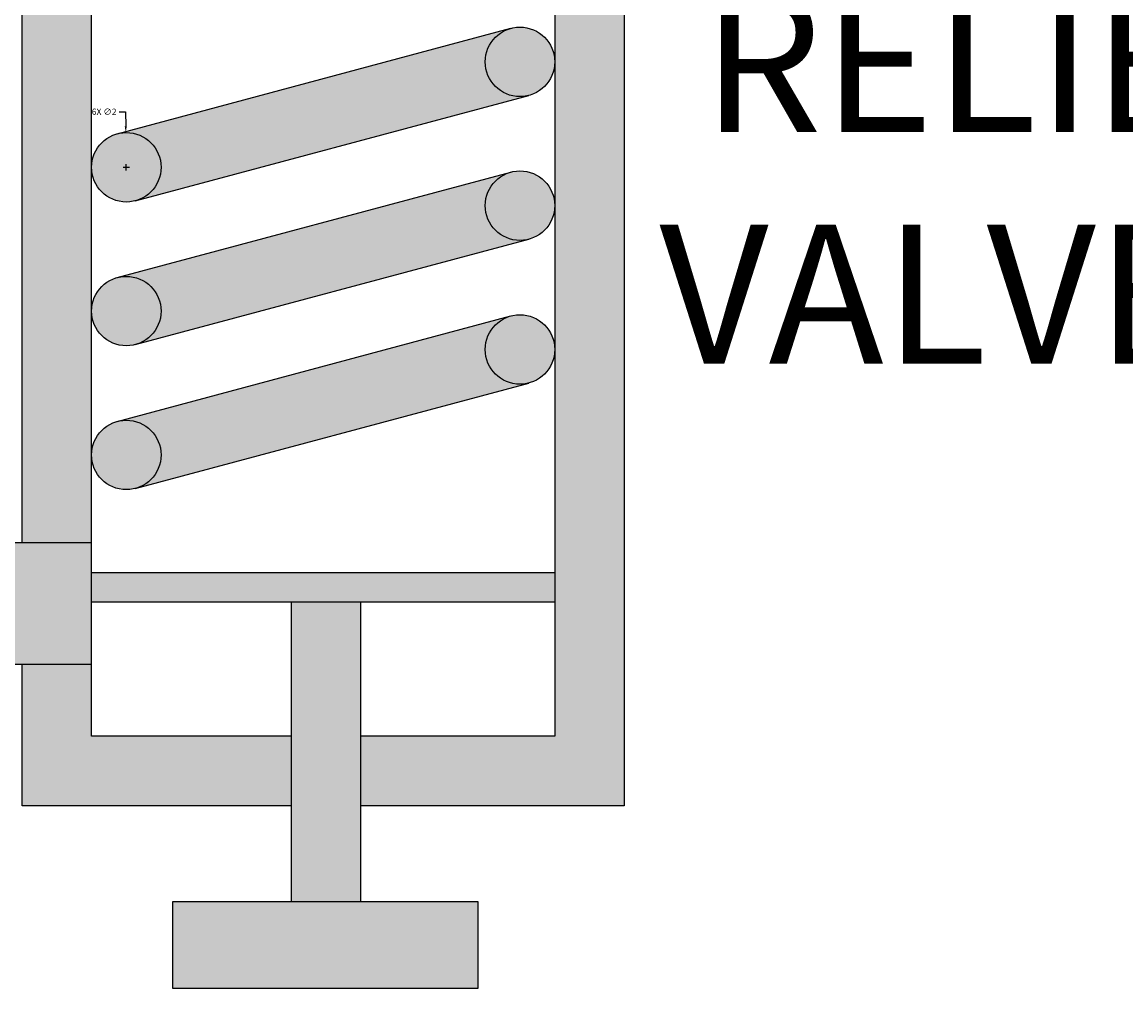
# Model space of a CAD drawing. Units: millimetres. Extents: x -11 to 280, y -4 to 208.
# Tile 23 of 55: x 119 to 150, y 61 to 89. Entities that reach past the tile are written whole.
import ezdxf

# ---------------------------------------------------------------- set-up
doc = ezdxf.new("R2010")
doc.units = ezdxf.units.MM
for name, color, linetype, lineweight in [('M-ANNO-TEXT', 7, 'Continuous', 18), ('M-DIMS', 2, 'Continuous', 18), ('M-HYDR-RETN', 7, 'Continuous', 25), ('M-HYDR-VALV', 7, 'Continuous', 25), ('M-HYDR-VALV-PATT', 252, 'Continuous', 13)]:
    doc.layers.add(name, color=color, linetype=linetype, lineweight=lineweight)
doc.layers.add('M-HYDR-RETN-PATT', color=114, linetype='Continuous', lineweight=13, true_color=0x139b48)
doc.styles.get("Standard").update_dxf_attribs({"font": 'arial.ttf'})
doc.dimstyles.get("Standard").update_dxf_attribs({"dimtxt": 0.18, "dimasz": 0.18, "dimexe": 0.18, "dimexo": 0.0625, "dimgap": 0.09, "dimtad": 0, "dimtih": 1, "dimtoh": 1, "dimdec": 4, "dimzin": 0, "dimdsep": 46, "dimtxsty": 'Standard', "dimcen": 0.09, "dimadec": 0, "dimazin": 0, "dimtfac": 1, "dimtdec": 4, "dimtofl": 0, "dimtmove": 0, "dimatfit": 3, "dimfxl": 1, "dimtolj": 1, "dimtzin": 0, "dimarcsym": 0})

# ---------------------------------------------------------------- blocks, each defined once
blk = doc.blocks.new('*D4')
at = {"layer": 'Defpoints', "color": 0, "transparency": 16777216}
for p in [(4.763, 84.426), (266.035, 51.733), (266.035, -3.415)]:
    blk.add_point(p, dxfattribs=at)
at = {"layer": 'M-DIMS', "color": 0, "lineweight": -2, "transparency": 16777216}
for p, q in [((4.763, 84.364), (4.763, -3.595)), ((266.035, 51.67), (266.035, -3.595)), ((4.943, -3.415), (134.934, -3.415)), ((265.855, -3.415), (135.864, -3.415))]:
    blk.add_line(p, q, dxfattribs=at)
at = {"layer": 'M-DIMS', "color": 0, "transparency": 16777216}
for points in [[(4.943, -3.385), (4.943, -3.445), (4.763, -3.415)], [(265.855, -3.385), (265.855, -3.445), (266.035, -3.415)]]:
    blk.add_solid(points, dxfattribs=at)
at = {"layer": 'M-DIMS', "color": 0, "transparency": 16777216, "insert": (135.399, -3.415), "char_height": 0.18, "attachment_point": 5}
blk.add_mtext('\\A1;261.27', dxfattribs=at)
blk = doc.blocks.new('*D5')
at = {"layer": 'Defpoints', "color": 0, "transparency": 16777216}
for p in [(24.759, 192.645), (-10.087, 11.435), (261.686, 11.435)]:
    blk.add_point(p, dxfattribs=at)
at = {"layer": 'M-DIMS', "color": 0, "lineweight": -2, "transparency": 16777216}
for p, q in [((24.696, 192.645), (-10.267, 192.645)), ((-10.087, 192.465), (-10.087, 102.222)), ((-10.087, 11.615), (-10.087, 101.858)), ((261.624, 11.435), (-10.267, 11.435))]:
    blk.add_line(p, q, dxfattribs=at)
at = {"layer": 'M-DIMS', "color": 0, "transparency": 16777216}
for points in [[(-10.117, 192.465), (-10.057, 192.465), (-10.087, 192.645)], [(-10.117, 11.615), (-10.057, 11.615), (-10.087, 11.435)]]:
    blk.add_solid(points, dxfattribs=at)
at = {"layer": 'M-DIMS', "color": 0, "transparency": 16777216, "insert": (-10.087, 102.04), "char_height": 0.18, "attachment_point": 5}
blk.add_mtext('\\A1;181.2', dxfattribs=at)
blk = doc.blocks.new('*D32')
at = {"layer": 'Defpoints', "color": 0, "transparency": 16777216}
for p in [(121.5, 86.206), (121.527, 84.206)]:
    blk.add_point(p, dxfattribs=at)
at = {"layer": 'M-DIMS', "color": 0, "lineweight": -2, "transparency": 16777216}
for p, q in [((121.312, 86.806), (121.492, 86.806)), ((121.492, 86.806), (121.497, 86.386)), ((121.424, 85.206), (121.604, 85.206)), ((121.514, 85.116), (121.514, 85.296))]:
    blk.add_line(p, q, dxfattribs=at)
at = {"layer": 'M-DIMS', "color": 0, "transparency": 16777216}
blk.add_solid([(121.527, 86.387), (121.467, 86.386), (121.5, 86.206)], dxfattribs=at)
at = {"layer": 'M-DIMS', "color": 0, "transparency": 16777216, "insert": (120.877, 86.806), "char_height": 0.18, "attachment_point": 5}
blk.add_mtext('\\A1;6X ∅2', dxfattribs=at)

msp = doc.modelspace()

# ---------------------------------------------------------------- hatches: boundary and pattern name
at = {"layer": 'M-HYDR-RETN-PATT'}
h = msp.add_hatch(color=256, dxfattribs=at)
h.set_gradient(color1=(19, 155, 72), color2=(19, 155, 72), tint=1)
h.paths.add_polyline_path([(17.9701, 159.0814), (29.2015, 159.0814), (29.2015, 162.5814), (14.4701, 162.5814), (14.4701, 98.0213), (17.9701, 98.0213)])
h.paths.add_polyline_path([(17.9701, 84.4261), (14.4701, 84.4261), (14.4701, 54.3099), (156.2446, 54.3099), (156.2446, 57.8099), (17.9701, 57.8099)])
h.paths.add_polyline_path([(120.5137, 74.3991), (17.9701, 74.3991), (17.9701, 70.8991), (120.5137, 70.8991)], flags=17)
h.paths.add_polyline_path([(184.7092, 75.04, 0.4142136), (179.7092, 80.04), (156.2446, 80.04), (156.2446, 57.8099), (156.2446, 54.3099), (156.2446, 43.5991), (159.7446, 43.5991), (159.7446, 57.8099), (159.7446, 76.54), (176.2092, 76.54, -0.4142136), (181.2092, 71.54), (181.2092, 57.8099), (159.7446, 57.8099), (159.7446, 54.3099), (184.7092, 54.3099)])
at = {"layer": 'M-HYDR-VALV-PATT'}
h = msp.add_hatch(color=256, dxfattribs=at)
h.set_gradient(color1=(153, 153, 0), color2=(153, 153, 0), tint=1)
h.paths.add_polyline_path([(135.8437, 96.4849), (128.8433, 96.4849), (128.8433, 94.4849), (133.8437, 94.4849), (133.8437, 68.8227), (128.2568, 68.8227), (128.2568, 66.8227), (135.8437, 66.8227)])
h.paths.add_polyline_path([(126.2568, 68.8227), (120.5137, 68.8227), (120.5137, 70.8991), (118.5137, 70.8991), (118.5137, 66.8227), (126.2568, 66.8227)])
h.paths.add_polyline_path([(120.5137, 94.4849), (125.3433, 94.4849), (125.3433, 96.4849), (118.5137, 96.4849), (118.5137, 74.3991), (120.5137, 74.3991)])
h.paths.add_polyline_path([(128.2568, 72.69), (126.2568, 72.69), (126.2568, 64.0664), (128.2568, 64.0664)])
h.paths.add_polyline_path([(131.6327, 64.0664), (122.8484, 64.0664), (122.8484, 61.5587), (131.6327, 61.5587)])
h.paths.add_polyline_path([(133.8437, 73.5419), (120.5137, 73.5419), (120.5137, 72.69), (133.8437, 72.69)])
h = msp.add_hatch(color=256, dxfattribs=at)
h.set_gradient(color1=(153, 27, 30), color2=(153, 27, 30), tint=1)
h.paths.add_polyline_path([(131.8437, 88.2421, -0.3394543), (132.5849, 89.208), (121.2548, 86.1721, -0.4931454), (122.5137, 85.2062, -0.3394543), (121.7725, 84.2403), (133.1025, 87.2762, -0.4931454)])
h.paths.add_polyline_path([(133.1025, 83.1351, -0.4931454), (131.8437, 84.101, -0.3394543), (132.5849, 85.0669), (121.2548, 82.031, -0.4931454), (122.5137, 81.0651, -0.3394543), (121.7725, 80.0992)])
h.paths.add_polyline_path([(133.1025, 78.994, -0.4931454), (131.8437, 79.9599, -0.3394543), (132.5849, 80.9258), (121.2548, 77.8899, -0.4931454), (122.5137, 76.924, -0.3394543), (121.7725, 75.9581)])
h.paths.add_polyline_path([(197.7905, 78.7098), (200.0003, 78.7098), (200.0003, 89.3873), (191.7745, 89.3873), (191.7745, 87.1776, -0.2439164)])
h.paths.add_polyline_path([(200.0003, 65.0638), (200.0003, 75.2098), (197.7325, 75.2098, -0.4135811), (184.7092, 66.0277), (184.7092, 65.0638)])
h.paths.add_polyline_path([(181.2092, 65.0638), (181.2092, 67.2471, -0.2598454), (175.3563, 76.54), (173.8038, 76.54), (173.8038, 65.0638)])
h.paths.add_polyline_path([(188.2745, 88.3022), (188.2745, 89.3873), (173.8038, 89.3873), (173.8038, 80.04), (175.7181, 80.04, -0.3816661)])
h = msp.add_hatch(color=256, dxfattribs=at)
h.set_gradient(color1=(41, 49, 137), color2=(34, 52, 110), tint=1)
h.paths.add_polyline_path([(120.5137, 85.2062, 1), (122.5137, 85.2062, 1)])
h.paths.add_polyline_path([(122.5137, 81.0651, 1), (120.5137, 81.0651, 1)])
h.paths.add_polyline_path([(120.5137, 76.924, 1), (122.5137, 76.924, 1)])
h.paths.add_polyline_path([(131.8437, 79.9599, 1), (133.8437, 79.9599, 1)])
h.paths.add_polyline_path([(133.8437, 84.101, 1), (131.8437, 84.101, 1)])
h.paths.add_polyline_path([(133.8437, 88.2421, 1), (131.8437, 88.2421, 1)])

# ---------------------------------------------------------------- linework, layer by layer
at = {"layer": 'M-HYDR-RETN'}
for points in [[(17.9701, 74.3991), (120.5137, 74.3991)], [(17.9701, 70.8991), (120.5137, 70.8991)]]:
    msp.add_lwpolyline(points, dxfattribs=at)
at = {"layer": 'M-HYDR-VALV'}
for p, q in [((121.2548, 86.1721), (132.5849, 89.208)), ((121.7725, 84.2403), (133.1025, 87.2762)), ((121.2548, 82.031), (132.5849, 85.0669)), ((121.7725, 80.0992), (133.1025, 83.1351)), ((121.2548, 77.8899), (132.5849, 80.9258)), ((121.7725, 75.9581), (133.1025, 78.994)), ((120.5137, 73.5419), (133.8437, 73.5419)), ((120.5137, 72.69), (133.8437, 72.69)), ((126.2568, 72.69), (126.2568, 64.0664)), ((128.2568, 72.69), (128.2568, 64.0664))]:
    msp.add_line(p, q, dxfattribs=at)
for points in [[(118.5137, 74.3991), (118.5137, 96.4849), (125.3433, 96.4849)], [(128.8433, 96.4849), (135.8437, 96.4849), (135.8437, 66.8227), (128.2568, 66.8227)], [(126.2568, 68.8227), (120.5137, 68.8227), (120.5137, 94.4849), (125.3433, 94.4849)], [(128.8433, 94.4849), (133.8437, 94.4849), (133.8437, 68.8227), (128.2568, 68.8227)], [(126.2568, 66.8227), (118.5137, 66.8227), (118.5137, 70.8991)]]:
    msp.add_lwpolyline(points, dxfattribs=at)
msp.add_lwpolyline([(122.8484, 64.0664), (131.6327, 64.0664), (131.6327, 61.5587), (122.8484, 61.5587)], close=True, dxfattribs=at)
for centre in [(132.8437, 88.2421), (121.5137, 85.2062), (132.8437, 84.101), (121.5137, 81.0651), (132.8437, 79.9599), (121.5137, 76.924)]:
    msp.add_circle(centre, 1, dxfattribs=at)

# ---------------------------------------------------------------- texts
at = {"layer": 'M-ANNO-TEXT', "insert": (136.8574, 96.8862), "char_height": 4, "attachment_point": 1}
msp.add_mtext_dynamic_manual_height_columns('PRESSURE\\P RELIEF\\PVALVE', width=63.617875, gutter_width=12.5, heights=[0], dxfattribs=at)

# ---------------------------------------------------------------- dimensions: what is measured, and where the dimension line sits
at = {"layer": 'M-DIMS'}
dim = msp.add_linear_dim(base=(-10.0865, 11.4346), p1=(24.7588, 192.645), p2=(261.6863, 11.4346), angle=90, dimstyle='Standard', override={"dimdec": 1, "dimlfac": 1, "dimrnd": 0, "dimzin": 0, "dimdsep": 46, "dimlunit": 2}, dxfattribs=at)
dim.commit()
dim.dimension.update_dxf_attribs({"geometry": '*D5', "text_midpoint": (-10.0865, 102.0398)})
dim = msp.add_diameter_dim_2p(p1=(121.5274, 84.2063), p2=(121.4999, 86.2061), text='6X <>', dimstyle='Standard', override={"dimdec": 0, "dimlfac": 1, "dimrnd": 0, "dimzin": 0, "dimdsep": 46, "dimlunit": 2}, dxfattribs=at)
dim.commit()
dim.dimension.update_dxf_attribs({"geometry": '*D32', "text_midpoint": (120.8766, 86.8061), "dimtype": 163})
dim = msp.add_linear_dim(base=(266.0352, -3.4154), p1=(4.7635, 84.4261), p2=(266.0352, 51.7328), dimstyle='Standard', override={"dimdec": 2, "dimlfac": 1, "dimrnd": 0, "dimzin": 0, "dimdsep": 46, "dimlunit": 2}, dxfattribs=at)
dim.commit()
dim.dimension.update_dxf_attribs({"geometry": '*D4', "text_midpoint": (135.3993, -3.4154)})

doc.saveas('drawing.dxf')
